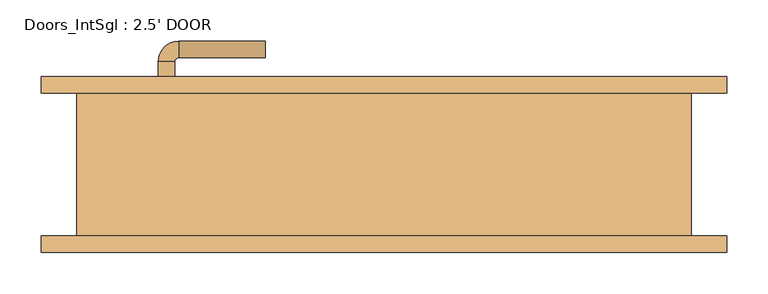
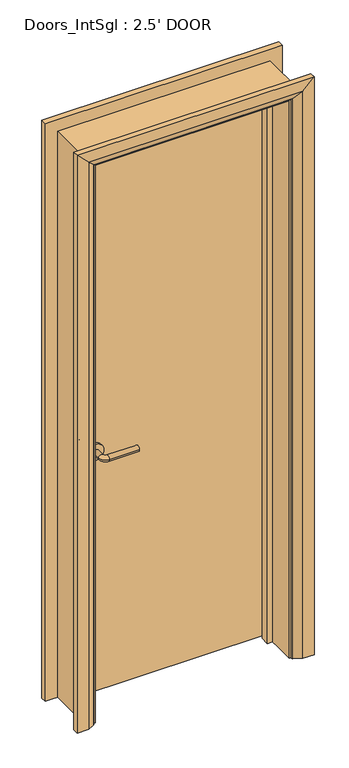
"""IFC4 building model written with IfcOpenShell, lengths in millimetres: door geometry, Doors_IntSgl : 2.5' DOOR."""

from ifc_helpers import new_model, si_unit, point, frame, frame_2d, origin, place, context, project, spatial, polyline, circle_curve, ellipse_curve, trimmed, segment, composite_curve, outline, extrude, faceted_brep, source, transform, mapped, element, save
from ifc_brep_helpers import plane_surface, cylinder_surface, revolved_surface, advanced_brep


def doors_intsgl_2_5_door_ce04bd24(model_context):
    return source(origin(), model_context, "Body", "SolidModel", [
        advanced_brep(
        [(-274.0, 40.868, 900.0), (-254.0, 40.868, 900.0), (-254.0, 10.868, 900.0), (-274.0, 10.868, 900.0), (-249.0, 5.868, 900.0), (-249.0, -14.132, 900.0), (-144.0, -14.132, 900.0), (-144.0, 5.868, 900.0)],
        [
            (0, 1, circle_curve(frame((-264.0, 40.868, 900.0), z_axis=(0.0, 1.0, 0.0), x_axis=(1.0, 0.0, 0.0)), 10.0)),
            (1, 0, circle_curve(frame((-264.0, 40.868, 900.0), z_axis=(0.0, 1.0, 0.0), x_axis=(1.0, 0.0, 0.0)), 10.0)),
            (1, 2),
            (2, 3, circle_curve(frame((-264.0, 10.868, 900.0), z_axis=(0.0, 1.0, 0.0), x_axis=(1.0, 0.0, 0.0)), 10.0)),
            (3, 0),
            (3, 2, circle_curve(frame((-264.0, 10.868, 900.0), z_axis=(0.0, 1.0, 0.0), x_axis=(1.0, 0.0, 0.0)), 10.0)),
            (4, 5, circle_curve(frame((-249.0, -4.132, 900.0), z_axis=(-1.0, 0.0, 0.0), x_axis=(0.0, 1.0, 0.0)), 10.0)),
            (5, 3, circle_curve(frame((-249.0, 10.868, 900.0), z_axis=(0.0, 0.0, -1.0), x_axis=(-1.0, 0.0, 0.0)), 25.0)),
            (2, 4, circle_curve(frame((-249.0, 10.868, 900.0), z_axis=(0.0, 0.0, 1.0), x_axis=(-1.0, 0.0, 0.0)), 5.0)),
            (5, 4, circle_curve(frame((-249.0, -4.132, 900.0), z_axis=(-1.0, 0.0, 0.0), x_axis=(0.0, 1.0, 0.0)), 10.0)),
            (6, 7, circle_curve(frame((-144.0, -4.132, 900.0), z_axis=(1.0, 0.0, 0.0), x_axis=(0.0, 1.0, 0.0)), 10.0)),
            (7, 6, circle_curve(frame((-144.0, -4.132, 900.0), z_axis=(1.0, 0.0, 0.0), x_axis=(0.0, 1.0, 0.0)), 10.0)),
            (4, 7),
            (6, 5),
        ],
        [
            plane_surface(frame((-264.0, 40.868, 900.0), z_axis=(0.0, 1.0, 0.0), x_axis=(0.0, 0.0, 1.0))),
            cylinder_surface(frame((-264.0, 40.868, 900.0), z_axis=(0.0, 1.0, 0.0), x_axis=(1.0, 0.0, 0.0)), 10.0),
            revolved_surface(trimmed(ellipse_curve(frame((-264.0, 10.868, 900.0), z_axis=(0.0, -1.0, 0.0), x_axis=(1.0, 0.0, 0.0)), 10.0, 10.0), [point((-274.0, 10.868, 900.0))], [point((-254.0, 10.868, 900.0))], True, "CARTESIAN"), (-249.0, 10.868, 900.0), (0.0, 0.0, -1.0)),
            revolved_surface(trimmed(ellipse_curve(frame((-264.0, 10.868, 900.0), z_axis=(0.0, -1.0, 0.0), x_axis=(1.0, 0.0, 0.0)), 10.0, 10.0), [point((-254.0, 10.868, 900.0))], [point((-274.0, 10.868, 900.0))], True, "CARTESIAN"), (-249.0, 10.868, 900.0), (0.0, 0.0, -1.0)),
            plane_surface(frame((-144.0, -4.132, 900.0), z_axis=(1.0, 0.0, 0.0), x_axis=(0.0, 0.0, 1.0))),
            cylinder_surface(frame((-249.0, -4.132, 900.0), z_axis=(-1.0, 0.0, 0.0), x_axis=(0.0, 1.0, 0.0)), 10.0),
        ],
        [
            (0, [[1, 2]]),
            (1, [[3, 4, 5, -2]]),
            (1, [[-5, 6, -3, -1]]),
            (2, [[7, 8, -4, 9]]),
            (3, [[10, -9, -6, -8]]),
            (4, [[11, 12]]),
            (5, [[13, -11, 14, -7]]),
            (5, [[-14, -12, -13, -10]]),
        ],
    ),
        extrude(outline(composite_curve([segment(trimmed(circle_curve(frame_2d((900.0, -266.5)), 30.0), [point((900.0, -296.5))], [point((900.0, -236.5))], False, "CARTESIAN"), True, "CONTINUOUS"), segment(trimmed(circle_curve(frame_2d((900.0, -266.5)), 30.0), [point((900.0, -236.5))], [point((900.0, -296.5))], False, "CARTESIAN"), True, "CONTINUOUS")], self_intersect=False)), frame((0.0, 40.868, 0.0), z_axis=(0.0, 1.0, 0.0), x_axis=(0.0, 0.0, 1.0)), (0.0, 0.0, 1.0), 8.0),
        advanced_brep(
        [(-274.0, 94.868, 900.0), (-254.0, 94.868, 900.0), (-274.0, 124.868, 900.0), (-254.0, 124.868, 900.0), (-249.0, 129.868, 900.0), (-249.0, 149.868, 900.0), (-144.0, 149.868, 900.0), (-144.0, 129.868, 900.0)],
        [
            (0, 1, circle_curve(frame((-264.0, 94.868, 900.0), z_axis=(0.0, -1.0, 0.0), x_axis=(1.0, 0.0, 0.0)), 10.0)),
            (1, 0, circle_curve(frame((-264.0, 94.868, 900.0), z_axis=(0.0, -1.0, 0.0), x_axis=(1.0, 0.0, 0.0)), 10.0)),
            (0, 2),
            (2, 3, circle_curve(frame((-264.0, 124.868, 900.0), z_axis=(0.0, -1.0, 0.0), x_axis=(1.0, 0.0, 0.0)), 10.0)),
            (3, 1),
            (3, 2, circle_curve(frame((-264.0, 124.868, 900.0), z_axis=(0.0, -1.0, 0.0), x_axis=(1.0, 0.0, 0.0)), 10.0)),
            (4, 3, circle_curve(frame((-249.0, 124.868, 900.0), z_axis=(0.0, 0.0, 1.0), x_axis=(-1.0, 0.0, 0.0)), 5.0)),
            (2, 5, circle_curve(frame((-249.0, 124.868, 900.0), z_axis=(0.0, 0.0, -1.0), x_axis=(-1.0, 0.0, 0.0)), 25.0)),
            (5, 4, circle_curve(frame((-249.0, 139.868, 900.0), z_axis=(-1.0, 0.0, 0.0), x_axis=(0.0, -1.0, 0.0)), 10.0)),
            (4, 5, circle_curve(frame((-249.0, 139.868, 900.0), z_axis=(-1.0, 0.0, 0.0), x_axis=(0.0, -1.0, 0.0)), 10.0)),
            (6, 7, circle_curve(frame((-144.0, 139.868, 900.0), z_axis=(1.0, 0.0, 0.0), x_axis=(0.0, -1.0, 0.0)), 10.0)),
            (7, 6, circle_curve(frame((-144.0, 139.868, 900.0), z_axis=(1.0, 0.0, 0.0), x_axis=(0.0, -1.0, 0.0)), 10.0)),
            (5, 6),
            (7, 4),
        ],
        [
            plane_surface(frame((-264.0, 94.868, 900.0), z_axis=(0.0, -1.0, 0.0), x_axis=(0.0, 0.0, 1.0))),
            cylinder_surface(frame((-264.0, 94.868, 900.0), z_axis=(0.0, -1.0, 0.0), x_axis=(1.0, 0.0, 0.0)), 10.0),
            revolved_surface(trimmed(ellipse_curve(frame((-264.0, 124.868, 900.0), z_axis=(0.0, -1.0, 0.0), x_axis=(1.0, 0.0, 0.0)), 10.0, 10.0), [point((-274.0, 124.868, 900.0))], [point((-254.0, 124.868, 900.0))], True, "CARTESIAN"), (-249.0, 124.868, 900.0), (0.0, 0.0, -1.0)),
            revolved_surface(trimmed(ellipse_curve(frame((-264.0, 124.868, 900.0), z_axis=(0.0, -1.0, 0.0), x_axis=(1.0, 0.0, 0.0)), 10.0, 10.0), [point((-254.0, 124.868, 900.0))], [point((-274.0, 124.868, 900.0))], True, "CARTESIAN"), (-249.0, 124.868, 900.0), (0.0, 0.0, -1.0)),
            plane_surface(frame((-144.0, 139.868, 900.0), z_axis=(1.0, 0.0, 0.0), x_axis=(0.0, 0.0, 1.0))),
            cylinder_surface(frame((-249.0, 139.868, 900.0), z_axis=(-1.0, 0.0, 0.0), x_axis=(0.0, -1.0, 0.0)), 10.0),
        ],
        [
            (0, [[1, 2]]),
            (1, [[-1, 3, 4, 5]]),
            (1, [[-2, -5, 6, -3]]),
            (2, [[7, -4, 8, 9]]),
            (3, [[-8, -6, -7, 10]]),
            (4, [[11, 12]]),
            (5, [[-9, 13, -12, 14]]),
            (5, [[-10, -14, -11, -13]]),
        ],
    ),
        extrude(outline(composite_curve([segment(trimmed(circle_curve(frame_2d((900.0, -266.5)), 30.0), [point((900.0, -296.5))], [point((900.0, -236.5))], False, "CARTESIAN"), True, "CONTINUOUS"), segment(trimmed(circle_curve(frame_2d((900.0, -266.5)), 30.0), [point((900.0, -236.5))], [point((900.0, -296.5))], False, "CARTESIAN"), True, "CONTINUOUS")], self_intersect=False)), frame((0.0, 86.868, 0.0), z_axis=(0.0, 1.0, 0.0), x_axis=(0.0, 0.0, 1.0)), (0.0, 0.0, 1.0), 8.0),
        extrude(outline(polyline([(339.0, 48.868), (-339.0, 48.868), (-339.0, 86.868), (339.0, 86.868), (339.0, 48.868)])), frame((0.0, 0.0, 8.0), z_axis=(0.0, 0.0, 1.0), x_axis=(1.0, 0.0, 0.0)), (0.0, 0.0, 1.0), 2060.0),
        advanced_brep(
        [(416.0, 106.868, 0.0), (416.0, 86.868, 0.0), (346.0, 86.868, 0.0), (350.0, 92.868, 0.0), (376.0, 106.868, 0.0), (416.0, 106.868, 2145.0), (416.0, 86.868, 2145.0), (-416.0, 86.868, 2145.0), (-416.0, 86.868, 0.0), (-346.0, 86.868, 0.0), (-346.0, 86.868, 2075.0), (346.0, 86.868, 2075.0), (350.0, 92.868, 2079.0), (376.0, 106.868, 2105.0), (-376.0, 106.868, 2105.0), (-376.0, 106.868, 0.0), (-416.0, 106.868, 0.0), (-416.0, 106.868, 2145.0), (-350.0, 92.868, 0.0), (-350.0, 92.868, 2079.0)],
        [
            (0, 1),
            (1, 2),
            (2, 3, circle_curve(frame((354.0, 85.868, 0.0), z_axis=(0.0, 0.0, -1.0), x_axis=(1.0, 0.0, 0.0)), 8.0622577)),
            (3, 4),
            (4, 0),
            (0, 5),
            (5, 6),
            (6, 1),
            (6, 7),
            (7, 8),
            (8, 9),
            (9, 10),
            (10, 11),
            (11, 2),
            (11, 12, ellipse_curve(frame((354.0, 85.868, 2083.0), z_axis=(0.7071067811865475, 0.0, -0.7071067811865475), x_axis=(-0.7071067811865474, 0.0, -0.7071067811865476)), 11.4017543, 8.0622577)),
            (12, 3),
            (12, 13),
            (13, 4),
            (13, 14),
            (14, 15),
            (15, 16),
            (16, 17),
            (17, 5),
            (7, 17),
            (16, 8),
            (15, 18),
            (18, 9, circle_curve(frame((-354.0, 85.868, 0.0), z_axis=(0.0, 0.0, -1.0), x_axis=(-1.0, 0.0, 0.0)), 8.0622577)),
            (19, 10, ellipse_curve(frame((-354.0, 85.868, 2083.0), z_axis=(-0.7071067811865475, 0.0, -0.7071067811865475), x_axis=(-0.7071067811865474, 0.0, 0.7071067811865476)), 11.4017543, 8.0622577)),
            (18, 19),
            (14, 19),
            (19, 12),
        ],
        [
            plane_surface(frame((346.0, 86.868, 0.0), z_axis=(0.0, 0.0, -1.0), x_axis=(0.0, -1.0, 0.0))),
            plane_surface(frame((416.0, 106.868, 0.0), z_axis=(1.0, 0.0, 0.0), x_axis=(0.0, 0.0, 1.0))),
            plane_surface(frame((416.0, 86.868, 0.0), z_axis=(0.0, -1.0, 0.0), x_axis=(0.0, 0.0, 1.0))),
            cylinder_surface(frame((354.0, 85.868, 0.0), z_axis=(0.0, 0.0, -1.0), x_axis=(1.0, 0.0, 0.0)), 8.0622577),
            plane_surface(frame((350.0, 92.868, 0.0), z_axis=(-0.4740998230350126, 0.880471099922178, 0.0), x_axis=(0.0, 0.0, 1.0))),
            plane_surface(frame((376.0, 106.868, 0.0), z_axis=(0.0, 1.0, 0.0), x_axis=(0.0, 0.0, 1.0))),
            plane_surface(frame((-416.0, 106.868, 2145.0), z_axis=(-1.0, 0.0, 0.0), x_axis=(0.0, 0.0, -1.0))),
            plane_surface(frame((-346.0, 86.868, 0.0), z_axis=(0.0, 0.0, -1.0), x_axis=(0.0, -1.0, 0.0))),
            cylinder_surface(frame((-354.0, 85.868, 2075.0), z_axis=(0.0, 0.0, 1.0), x_axis=(-1.0, 0.0, 0.0)), 8.0622577),
            plane_surface(frame((-350.0, 92.868, 2079.0), z_axis=(0.47409982303501824, 0.8804710999221749, 0.0), x_axis=(0.0, 0.0, -1.0))),
            plane_surface(frame((416.0, 106.868, 2145.0), z_axis=(0.0, 0.0, 1.0), x_axis=(-1.0, 0.0, 0.0))),
            cylinder_surface(frame((346.0, 85.868, 2083.0), z_axis=(1.0, 0.0, 0.0), x_axis=(0.0, 0.0, 1.0)), 8.0622577),
            plane_surface(frame((350.0, 92.868, 2079.0), z_axis=(0.0, 0.8804710999221764, -0.4740998230350154), x_axis=(-1.0, 0.0, 0.0))),
        ],
        [
            (0, [[1, 2, 3, 4, 5]]),
            (1, [[-1, 6, 7, 8]]),
            (2, [[-2, -8, 9, 10, 11, 12, 13, 14]]),
            (3, [[-3, -14, 15, 16]]),
            (4, [[-4, -16, 17, 18]]),
            (5, [[-5, -18, 19, 20, 21, 22, 23, -6]]),
            (6, [[24, -22, 25, -10]]),
            (7, [[-21, 26, 27, -11, -25]]),
            (8, [[28, -12, -27, 29]]),
            (9, [[30, -29, -26, -20]]),
            (10, [[-7, -23, -24, -9]]),
            (11, [[-15, -13, -28, 31]]),
            (12, [[-17, -31, -30, -19]]),
        ],
    ),
        extrude(outline(polyline([(0.0, -341.0), (0.0, -322.0), (2051.0, -322.0), (2051.0, 322.0), (0.0, 322.0), (0.0, 341.0), (2070.0, 341.0), (2070.0, -341.0), (0.0, -341.0)])), frame((0.0, 14.868, 0.0), z_axis=(0.0, 1.0, 0.0), x_axis=(0.0, 0.0, 1.0)), (0.0, 0.0, 1.0), 32.0),
        advanced_brep(
        [(-416.0, -106.868, 0.0), (-416.0, -86.868, 0.0), (-346.0, -86.868, 0.0), (-350.0, -92.868, 0.0), (-376.0, -106.868, 0.0), (-416.0, -106.868, 2145.0), (-416.0, -86.868, 2145.0), (-346.0, -86.868, 2075.0), (-350.0, -92.868, 2079.0), (-376.0, -106.868, 2105.0), (416.0, -106.868, 0.0), (376.0, -106.868, 0.0), (350.0, -92.868, 0.0), (346.0, -86.868, 0.0), (416.0, -86.868, 0.0), (416.0, -106.868, 2145.0), (376.0, -106.868, 2105.0), (350.0, -92.868, 2079.0), (346.0, -86.868, 2075.0), (416.0, -86.868, 2145.0)],
        [
            (0, 1),
            (1, 2),
            (2, 3, circle_curve(frame((-354.0, -85.868, 0.0), z_axis=(0.0, 0.0, -1.0), x_axis=(-1.0, 0.0, 0.0)), 8.0622577)),
            (3, 4),
            (4, 0),
            (0, 5),
            (5, 6),
            (6, 1),
            (6, 7),
            (7, 2),
            (7, 8, ellipse_curve(frame((-354.0, -85.868, 2083.0), z_axis=(-0.7071067811865475, 0.0, -0.7071067811865475), x_axis=(0.7071067811865474, 0.0, -0.7071067811865476)), 11.4017543, 8.0622577)),
            (8, 3),
            (8, 9),
            (9, 4),
            (9, 5),
            (10, 11),
            (11, 12),
            (12, 13, circle_curve(frame((354.0, -85.868, 0.0), z_axis=(0.0, 0.0, -1.0), x_axis=(1.0, 0.0, 0.0)), 8.0622577)),
            (13, 14),
            (14, 10),
            (15, 16),
            (16, 11),
            (10, 15),
            (16, 17),
            (17, 12),
            (17, 18, ellipse_curve(frame((354.0, -85.868, 2083.0), z_axis=(0.7071067811865475, 0.0, -0.7071067811865475), x_axis=(0.7071067811865474, 0.0, 0.7071067811865476)), 11.4017543, 8.0622577)),
            (18, 13),
            (18, 19),
            (19, 14),
            (19, 15),
            (5, 15),
            (19, 6),
            (18, 7),
            (17, 8),
            (16, 9),
        ],
        [
            plane_surface(frame((-346.0, -159.6690989, 0.0), z_axis=(0.0, 0.0, -1.0), x_axis=(1.0, 0.0, 0.0))),
            plane_surface(frame((-416.0, -106.868, 0.0), z_axis=(-1.0, 0.0, 0.0), x_axis=(0.0, 0.0, 1.0))),
            plane_surface(frame((-416.0, -86.868, 0.0), z_axis=(0.0, 1.0, 0.0), x_axis=(0.0, 0.0, 1.0))),
            cylinder_surface(frame((-354.0, -85.868, 0.0), z_axis=(0.0, 0.0, -1.0), x_axis=(-1.0, 0.0, 0.0)), 8.0622577),
            plane_surface(frame((-350.0, -92.868, 0.0), z_axis=(0.4740998230350183, -0.8804710999221749, 0.0), x_axis=(0.0, 0.0, 1.0))),
            plane_surface(frame((-376.0, -106.868, 0.0), z_axis=(0.0, -1.0, 0.0), x_axis=(0.0, 0.0, 1.0))),
            plane_surface(frame((346.0, -159.6690989, 0.0), z_axis=(0.0, 0.0, -1.0), x_axis=(-1.0, 0.0, 0.0))),
            plane_surface(frame((376.0, -106.868, 2105.0), z_axis=(0.0, -1.0, 0.0), x_axis=(0.0, 0.0, -1.0))),
            plane_surface(frame((350.0, -92.868, 2079.0), z_axis=(-0.4740998230350183, -0.8804710999221749, 0.0), x_axis=(0.0, 0.0, -1.0))),
            cylinder_surface(frame((354.0, -85.868, 2075.0), z_axis=(0.0, 0.0, 1.0), x_axis=(1.0, 0.0, 0.0)), 8.0622577),
            plane_surface(frame((416.0, -86.868, 2145.0), z_axis=(0.0, 1.0, 0.0), x_axis=(0.0, 0.0, -1.0))),
            plane_surface(frame((416.0, -106.868, 2145.0), z_axis=(1.0, 0.0, 0.0), x_axis=(0.0, 0.0, -1.0))),
            plane_surface(frame((-416.0, -106.868, 2145.0), z_axis=(0.0, 0.0, 1.0), x_axis=(1.0, 0.0, 0.0))),
            plane_surface(frame((-416.0, -86.868, 2145.0), z_axis=(0.0, 1.0, 0.0), x_axis=(1.0, 0.0, 0.0))),
            cylinder_surface(frame((-346.0, -85.868, 2083.0), z_axis=(-1.0, 0.0, 0.0), x_axis=(0.0, 0.0, 1.0)), 8.0622577),
            plane_surface(frame((-350.0, -92.868, 2079.0), z_axis=(0.0, -0.8804710999221749, -0.4740998230350183), x_axis=(1.0, 0.0, 0.0))),
            plane_surface(frame((-376.0, -106.868, 2105.0), z_axis=(0.0, -1.0, 0.0), x_axis=(1.0, 0.0, 0.0))),
        ],
        [
            (0, [[1, 2, 3, 4, 5]]),
            (1, [[-1, 6, 7, 8]]),
            (2, [[-2, -8, 9, 10]]),
            (3, [[-3, -10, 11, 12]]),
            (4, [[-4, -12, 13, 14]]),
            (5, [[-5, -14, 15, -6]]),
            (6, [[16, 17, 18, 19, 20]]),
            (7, [[21, 22, -16, 23]]),
            (8, [[24, 25, -17, -22]]),
            (9, [[26, 27, -18, -25]]),
            (10, [[28, 29, -19, -27]]),
            (11, [[30, -23, -20, -29]]),
            (12, [[-7, 31, -30, 32]]),
            (13, [[-9, -32, -28, 33]]),
            (14, [[-11, -33, -26, 34]]),
            (15, [[-13, -34, -24, 35]]),
            (16, [[-15, -35, -21, -31]]),
        ],
    ),
        faceted_brep([(-341.0, 86.868, 0.0), (-341.0, -86.868, 0.0), (-373.0, -86.868, 0.0), (-373.0, 86.868, 0.0), (-341.0, 86.868, 2070.0), (-341.0, -86.868, 2070.0), (-373.0, -86.868, 2102.0), (-373.0, 86.868, 2102.0), (341.0, 86.868, 0.0), (373.0, 86.868, 0.0), (373.0, -86.868, 0.0), (341.0, -86.868, 0.0), (341.0, 86.868, 2070.0), (373.0, 86.868, 2102.0), (373.0, -86.868, 2102.0), (341.0, -86.868, 2070.0)], [[[0, 1, 2, 3]], [[1, 0, 4, 5]], [[2, 1, 5, 6]], [[3, 2, 6, 7]], [[0, 3, 7, 4]], [[8, 9, 10, 11]], [[12, 13, 9, 8]], [[13, 14, 10, 9]], [[14, 15, 11, 10]], [[15, 12, 8, 11]], [[5, 4, 12, 15]], [[6, 5, 15, 14]], [[7, 6, 14, 13]], [[4, 7, 13, 12]]]),
    ])


if __name__ == "__main__":
    model = new_model("IFC4")
    model_context = context("Model", 3, world=origin())
    ifc_project = project(units=[si_unit("LENGTHUNIT", "METRE", prefix="MILLI")], contexts=[model_context])
    site = spatial("IfcSite", under=ifc_project)
    building = spatial("IfcBuilding", under=site)
    placement = place(None, origin())
    doors_intsgl_2_5_door_shape = doors_intsgl_2_5_door_ce04bd24(model_context)
    element("IfcDoor", 1, ObjectType="Doors_IntSgl : 2.5' DOOR", at=placement, inside=building, context=model_context, shape_type="MappedRepresentation", body=[
        mapped(doors_intsgl_2_5_door_shape, transform((0.0, 0.0, 0.0), x_axis=(1.0, 0.0, 0.0), y_axis=(0.0, 1.0, 0.0), z_axis=(0.0, 0.0, 1.0))),
    ])
    save(model, "model.ifc")

# Revit data of these elements
# Type "Doors_IntSgl : 2.5' DOOR"
#   Type Mark = "47"
#   Type Comments = "Internal Single"
#   Operation = "SingleSwingRight"
#   Manufacturer = "Revit"
#   Keynote = "L20"
#   Description = "Internal Single Door"
#   Analytic Construction = "Metal"
#   UnderCut = 0.026247 ft
#   Tolerance = 0.006562 ft
#   Thickness = 0.124672 ft
#   Thermal Resistance (R) = 0.270117 (m²·K)/W
#   Structural Tolerance = 0.026247 ft
#   StopDepth = 0.104987 ft
#   Stop Thickness = 0.062336 ft
#   Rough Width = 2.5 ft
#   Rough Height = 6.922572 ft
#   Height to Top Lock Rail = 3.28084 ft
#   Heat Transfer Coefficient (U) = 3.7021 W/(m²·K)
#   Handle Z Distance = 2.952756 ft
#   Handle X Distance = 0.246063 ft
#   Frame Thickness = 0.104987 ft
#   Door Panel Width = 2.224409 ft
#   Door Panel Thickness = 0.124672 ft
#   Door Panel Offset = 0.0 ft
#   Height = 6.922572 ft
#   Width = 2.5 ft
#   Door Panel Height = 6.75853 ft
#   Architrave Setback = 0.016404 ft
#   Vis - Ironmongery = yes
#   Material Ironmongery = Door - Handle
#   Material Frame = Door - Frame/Mullion (1)
#   Material Door = Door - Panel
#   Material Architrave = Door - Architrave
#   Visual Light Transmittance = 0
#   Solar Heat Gain Coefficient = 0
#   Function = (empty or 0)
#   Wall Closure = (empty or 0)
# Element 1 (IfcDoor, "Doors_IntSgl : 2.5' DOOR")
#   Materials on its faces: "Door - Architrave", "Door - Handle", "Door - Frame/Mullion (1)", "Door - Panel"
# Materials
#   "Door - Handle": colour RGB 0 0 0, transparency 0, Keynote = "P21", Cost = 0
#   "Door - Frame/Mullion (1)": class "Wood", colour RGB 212 179 113, transparency 0, Keynote = "L20", Cost = 0
#   "Door - Panel": class "Wood", colour RGB 210 159 95, transparency 0, Keynote = "L20", Cost = 0
#   "Door - Architrave": class "Wood", colour RGB 154 90 5, transparency 0, Keynote = "P20", Cost = 0
